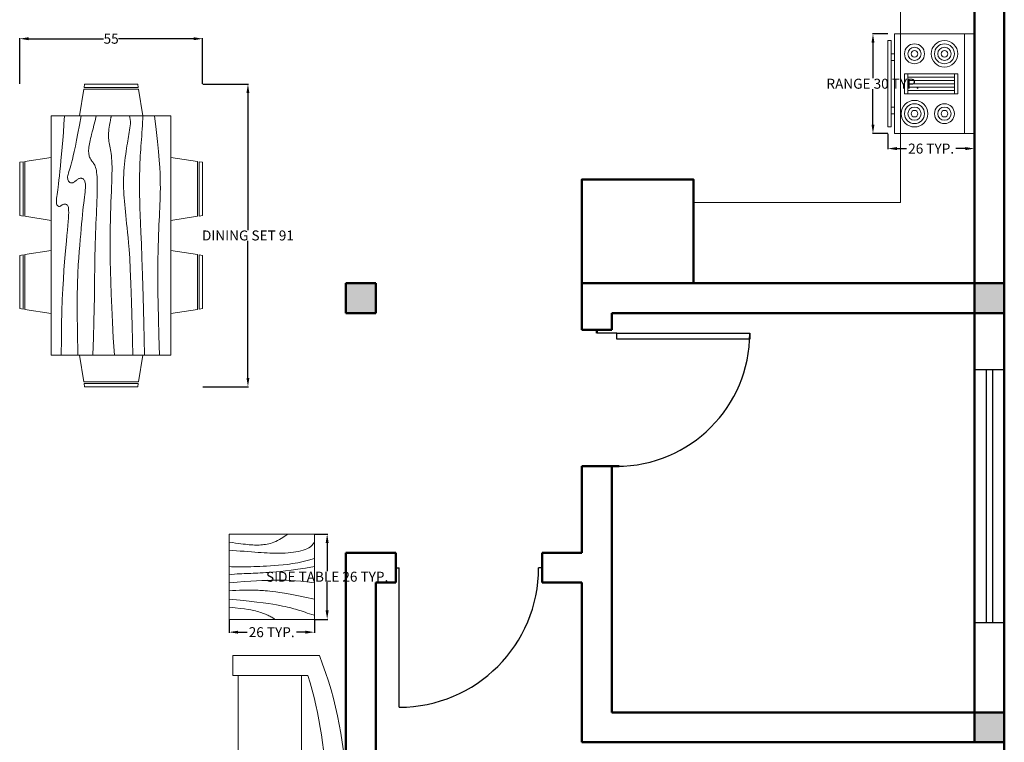
# Model space of a CAD drawing. Units: inches. Extents: x 13 to 1693, y -7 to 1519.
# Tile 3 of 10: x 387 to 683, y 360 to 577. Entities that reach past the tile are written whole.
import ezdxf

# ---------------------------------------------------------------- set-up
doc = ezdxf.new("R2010")
doc.units = ezdxf.units.IN
doc.header["$MEASUREMENT"] = 0
for name, color, linetype, lineweight in [('A-ANNO-DIMS', 2, 'Continuous', 18), ('A-DOOR', 4, 'Continuous', 25), ('A-FLOR-CASE', 5, 'Continuous', 18), ('A-FLOR-FIXT', 9, 'Continuous', 18), ('A-FURN', 8, 'Continuous', 18), ('A-GLAZ', 4, 'Continuous', 25), ('A-WALL', 7, 'Continuous', 50), ('A-WALL-PATT', 8, 'Continuous', 13)]:
    doc.layers.add(name, color=color, linetype=linetype, lineweight=lineweight)
doc.styles.get("Standard").update_dxf_attribs({"font": 'arial.ttf'})
doc.dimstyles.get("Standard").update_dxf_attribs({"dimtxt": 3, "dimasz": 2.68, "dimexe": 0.18, "dimexo": 0.0625, "dimgap": 0.09, "dimtad": 0, "dimtih": 1, "dimtoh": 1, "dimdec": 0, "dimzin": 0, "dimdsep": 46, "dimlunit": 3, "dimtxsty": 'Standard', "dimcen": 0.09, "dimadec": 0, "dimazin": 0, "dimtfac": 1, "dimtdec": 0, "dimtofl": 0, "dimtmove": 0, "dimatfit": 3, "dimfxl": 1, "dimtolj": 1, "dimtzin": 0, "dimarcsym": 0})

# ---------------------------------------------------------------- blocks, each defined once
blk = doc.blocks.new('*U6')
for p, q in [((0, 0), (0, -6)), ((40, 0), (40, -6))]:
    blk.add_line(p, q)
blk.add_lwpolyline([(0, 0), (0, 40), (1.75, 40), (1.75, 0)], close=True)
blk.add_arc((0, 0), 40, 0, 90)
blk = doc.blocks.new('Table - Square Woodgrain 42 x 42 in.')
blk.add_line((0, -42), (42, -42))
for points in [[(0, -4), (1.704, -4.2172), (3.2358, -4.4188), (4.615, -4.604), (5.8615, -4.7721), (6.9951, -4.9224), (8.0357, -5.0541), (9.0031, -5.1667), (9.9171, -5.2594), (10.7951, -5.3316), (11.6445, -5.3836), (12.4702, -5.4157), (13.277, -5.4283), (14.0698, -5.4217), (14.8535, -5.3964), (15.6331, -5.3526), (16.4133, -5.2908), (17.1986, -5.2103), (17.9913, -5.1062), (18.793, -4.9727), (19.6056, -4.8038), (20.4307, -4.5937), (21.2701, -4.3365), (22.1256, -4.0262), (22.9989, -3.6571), (23.888, -3.2272), (24.7756, -2.7516), (25.6408, -2.2491), (26.4624, -1.7387), (27.2195, -1.2395), (27.891, -0.7703), (28.456, -0.3501), (28.8934, 0.002)], [(0, -42), (0, 0), (42, 0), (42, -42)], [(0, -8), (1.8203, -8.1001), (3.6741, -8.2149), (5.5411, -8.3408), (7.4011, -8.4741), (9.2339, -8.6112), (11.0193, -8.7484), (12.7371, -8.8821), (14.3671, -9.0086), (15.8954, -9.1246), (17.3337, -9.2278), (18.6997, -9.3159), (20.0116, -9.387), (21.2871, -9.4389), (22.5442, -9.4696), (23.8008, -9.477), (25.0749, -9.459), (26.3791, -9.4137), (27.7049, -9.3403), (29.0383, -9.2382), (30.3655, -9.1068), (31.6728, -8.9455), (32.9461, -8.7535), (34.1717, -8.5304), (35.3358, -8.2756), (36.4268, -7.9863), (37.443, -7.6521), (38.3849, -7.2603), (39.253, -6.7986), (40.048, -6.2542), (40.7705, -5.6147), (41.421, -4.8674), (42, -4)], [(42, -12), (39.1784, -12.8621), (36.4519, -13.5654), (33.8246, -14.1294), (31.3004, -14.5731), (28.8832, -14.9161), (26.577, -15.1775), (24.3858, -15.3768), (22.3136, -15.5332), (20.3622, -15.6632), (18.5254, -15.7718), (16.7947, -15.8612), (15.1618, -15.9338), (13.6183, -15.9916), (12.1558, -16.0369), (10.7659, -16.0718), (9.4403, -16.0987), (8.1703, -16.1191), (6.9461, -16.1325), (5.7577, -16.1377), (4.595, -16.1335), (3.4479, -16.1188), (2.3064, -16.0924), (1.1604, -16.0532), (0, -16)], [(42, -16), (37.6529, -16.7365), (33.8802, -17.329), (30.6179, -17.7961), (27.8015, -18.1561), (25.3668, -18.4275), (23.2497, -18.6288), (21.3859, -18.7785), (19.7111, -18.8949), (18.1693, -18.9939), (16.7375, -19.0795), (15.401, -19.1534), (14.1449, -19.217), (12.9544, -19.2717), (11.8148, -19.3191), (10.7113, -19.3606), (9.6291, -19.3976), (8.5534, -19.4323), (7.47, -19.4689), (6.3643, -19.5122), (5.222, -19.5672), (4.0288, -19.6386), (2.7703, -19.7313), (1.4321, -19.8501), (0, -20)], [(0, -24), (3.9243, -23.6805), (7.4766, -23.4138), (10.6891, -23.1954), (13.5943, -23.0205), (16.2247, -22.8847), (18.6125, -22.7832), (20.7903, -22.7116), (22.7903, -22.6651), (24.6563, -22.642), (26.4764, -22.6507), (28.35, -22.7024), (30.3766, -22.8084), (32.6555, -22.98), (35.2861, -23.2283), (38.3678, -23.5645), (42, -24)], [(42, -32), (37.392, -31.017), (33.4585, -30.2231), (30.1291, -29.5949), (27.3334, -29.109), (25.0009, -28.742), (23.0612, -28.4707), (21.4439, -28.2716), (20.0786, -28.1215), (18.8998, -28.0002), (17.8609, -27.9014), (16.9206, -27.8219), (16.0371, -27.7588), (15.1691, -27.709), (14.2748, -27.6693), (13.3128, -27.6368), (12.2415, -27.6083), (11.0295, -27.5824), (9.6867, -27.5643), (8.233, -27.5608), (6.6884, -27.5787), (5.0728, -27.6248), (3.4062, -27.7058), (1.7086, -27.8286), (0, -28)], [(0, -32), (5.4026, -32.5358), (9.9494, -33.019), (13.7424, -33.4553), (16.8834, -33.8505), (19.4743, -34.2106), (21.6171, -34.5413), (23.4136, -34.8486), (24.9657, -35.1382), (26.3614, -35.4156), (27.6332, -35.6841), (28.7995, -35.9467), (29.8788, -36.2064), (30.8897, -36.4661), (31.8507, -36.7288), (32.7802, -36.9973), (33.6968, -37.2747), (34.6175, -37.5635), (35.5531, -37.8651), (36.5128, -38.1805), (37.506, -38.5108), (38.5421, -38.8568), (39.6302, -39.2197), (40.7797, -39.6004), (42, -40)], [(0, -36), (3.0098, -36.2857), (5.5354, -36.5643), (7.6368, -36.8359), (9.374, -37.1009), (10.807, -37.3597), (11.9957, -37.6126), (13.0002, -37.8599), (13.8804, -38.102), (14.6874, -38.3393), (15.4365, -38.5729), (16.1338, -38.8041), (16.7858, -39.0341), (17.3987, -39.264), (17.9787, -39.4952), (18.5322, -39.7288), (19.0655, -39.9662), (19.5832, -40.2081), (20.0842, -40.4544), (20.5657, -40.7046), (21.0249, -40.9581), (21.459, -41.2144), (21.8653, -41.4731), (22.2409, -41.7335), (22.5831, -41.9951)]]:
    blk.add_lwpolyline(points)
blk = doc.blocks.new('Sofa - Roundback 7 ft.')
for p, q in [((-12.00002, -32.4421), (-12.00003, -6.5971)), ((11.99997, -32.4421), (11.99998, -6.5971)), ((-36.000027, -34), (-36.000027, -11.4696)), ((35.99998, -34), (35.99998, -11.4696)), ((-35.999844, -13.3819), (35.9998, -13.3819)), ((-36.000027, -32.4421), (35.99998, -32.4421))]:
    blk.add_line(p, q)
for points in [[(-36.000027, -34), (-42.000027, -34), (-42.000027, -8)], [(41.99998, -8), (41.99998, -34), (35.99998, -34)]]:
    blk.add_lwpolyline(points)
for centre, radius, start, end in [((0, -114.25), 114.25, 68.43141, 111.5686), ((-0.00001, -127.1968), 121.1968, 72.72033, 107.2797)]:
    blk.add_arc(centre, radius, start, end)
blk = doc.blocks.new('Dining Set - 36 x 72 in.')
for p, q in [((-22, 27.5), (-22.1562, 26.50042)), ((-22, 27.5), (-6, 27.5)), ((-5.8437, 26.49966), (-6, 27.5)), ((6, 27.5), (5.8438, 26.50042)), ((6, 27.5), (22, 27.5)), ((22.1563, 26.49966), (22, 27.5)), ((-22.2343, 26.00059), (-23.4847, 17.99762)), ((-22.2304, 26), (-5.7608, 26)), ((-5.8416, 26.5), (-22.1534, 26.5)), ((-4.5152, 17.99762), (-5.7655, 25.99926)), ((5.7657, 26.00059), (4.5153, 17.99762)), ((5.7696, 26), (22.2392, 26)), ((22.1584, 26.5), (5.8466, 26.5)), ((23.4848, 17.99762), (22.2345, 25.99926)), ((36, 18), (-36, 18)), ((-36, 18), (-36, -18)), ((36, -18), (36, 18)), ((-44.0006, 8.23428), (-35.9976, 9.48474)), ((44.0006, 8.23428), (35.9976, 9.48474)), ((-45.5, 8), (-44.5004, 8.15617)), ((-45.5, 8), (-45.5, -8)), ((-44.5, -8.15843), (-44.5, 8.15338)), ((-44, 8.23041), (-44, -8.23915)), ((44, 8.23041), (44, -8.23915)), ((44.5, -8.15843), (44.5, 8.15338)), ((45.5, 8), (44.5005, 8.15617)), ((45.5, 8), (45.5, -8)), ((-44.4997, -8.15631), (-45.5, -8)), ((-35.9976, -9.48476), (-43.9993, -8.2345)), ((35.9976, -9.48476), (43.9993, -8.2345)), ((44.4997, -8.15631), (45.5, -8)), ((-36, -18), (36, -18)), ((-22.2343, -26.0006), (-23.4847, -17.99762)), ((-4.5152, -17.99762), (-5.7655, -25.99928)), ((5.7657, -26.0006), (4.5153, -17.99762)), ((23.4848, -17.99762), (22.2345, -25.99928)), ((-22.2304, -26), (-5.7608, -26)), ((-22, -27.5), (-22.1562, -26.50044)), ((-5.8416, -26.5), (-22.1534, -26.5)), ((-5.8437, -26.49967), (-6, -27.5)), ((5.7696, -26), (22.2392, -26)), ((6, -27.5), (5.8438, -26.50044)), ((22.1584, -26.5), (5.8466, -26.5)), ((22.1563, -26.49967), (22, -27.5)), ((-22, -27.5), (-6, -27.5)), ((6, -27.5), (22, -27.5))]:
    blk.add_line(p, q)
for points in [[(-36, 15), (-31.1772, 14.97754), (-26.8079, 14.91406), (-22.8538, 14.81543), (-19.276, 14.6875), (-16.0362, 14.53613), (-13.0957, 14.36718), (-10.4159, 14.18652), (-7.9583, 14), (-5.6904, 13.81315), (-3.6035, 13.63021), (-1.6954, 13.45508), (0.0365, 13.29166), (1.5945, 13.14388), (2.9811, 13.01562), (4.1988, 12.9108), (5.25, 12.83333), (6.1393, 12.78613), (6.8802, 12.76823), (7.4883, 12.77767), (7.9792, 12.8125), (8.3685, 12.87077), (8.6719, 12.95052), (8.9049, 13.0498), (9.0833, 13.16666), (9.2205, 13.29899), (9.3216, 13.44401), (9.3895, 13.59879), (9.4271, 13.76041), (9.4373, 13.92594), (9.4232, 14.09245), (9.3875, 14.257), (9.3333, 14.41666), (9.2638, 14.56917), (9.1836, 14.71484), (9.0975, 14.85465), (9.0104, 14.98958), (8.9272, 15.1206), (8.8529, 15.2487), (8.7922, 15.37483), (8.75, 15.5), (8.7305, 15.62467), (8.7344, 15.74739), (8.7617, 15.86621), (8.8125, 15.97916), (8.8867, 16.08431), (8.9844, 16.17968), (9.1055, 16.26334), (9.25, 16.33333), (9.4189, 16.38802), (9.6172, 16.42708), (9.8506, 16.45052), (10.125, 16.45833), (10.4463, 16.45052), (10.8203, 16.42708), (11.2529, 16.38802), (11.75, 16.33333), (12.3184, 16.26318), (12.9694, 16.17838), (13.7151, 16.07991), (14.5677, 15.96875), (15.5395, 15.84586), (16.6426, 15.71224), (17.8893, 15.56884), (19.2917, 15.41666), (20.859, 15.25667), (22.5879, 15.08984), (24.4721, 14.91715), (26.5052, 14.73958), (28.6809, 14.5581), (30.9929, 14.3737), (33.4347, 14.18733), (36, 14)], [(-36, 10), (-28.9766, 10.14274), (-23.1725, 10.20442), (-18.4241, 10.19775), (-14.5677, 10.13541), (-11.4399, 10.03011), (-8.877, 9.89453), (-6.7154, 9.74137), (-4.7917, 9.58333), (-2.9698, 9.43082), (-1.2246, 9.28515), (0.4415, 9.14534), (2.026, 9.01041), (3.5266, 8.87939), (4.9408, 8.7513), (6.266, 8.62516), (7.5, 8.5), (8.6411, 8.37549), (9.6914, 8.2539), (10.6538, 8.13818), (11.5312, 8.03125), (12.3267, 7.93603), (13.043, 7.85547), (13.6831, 7.79248), (14.25, 7.75), (14.7471, 7.7303), (15.1797, 7.73307), (15.5537, 7.75732), (15.875, 7.80208), (16.1494, 7.86637), (16.3828, 7.94922), (16.5811, 8.04964), (16.75, 8.16666), (16.8944, 8.29915), (17.0143, 8.44531), (17.1089, 8.60319), (17.1771, 8.77083), (17.218, 8.94629), (17.2305, 9.1276), (17.2137, 9.31282), (17.1667, 9.5), (17.0895, 9.6875), (16.987, 9.875), (16.8649, 10.0625), (16.7292, 10.25), (16.5856, 10.4375), (16.4401, 10.625), (16.2985, 10.8125), (16.1667, 11), (16.05, 11.18733), (15.9518, 11.3737), (15.8752, 11.5581), (15.8229, 11.73958), (15.798, 11.91715), (15.8034, 12.08984), (15.842, 12.25667), (15.9167, 12.41666), (16.0295, 12.56836), (16.1784, 12.70833), (16.3605, 12.83268), (16.5729, 12.9375), (16.8127, 13.01888), (17.0768, 13.07291), (17.3625, 13.0957), (17.6667, 13.08333), (17.9894, 13.03312), (18.3418, 12.94726), (18.7382, 12.82918), (19.1927, 12.68229), (19.7195, 12.51001), (20.3327, 12.31575), (21.0465, 12.10294), (21.875, 11.875), (22.8357, 11.63354), (23.959, 11.37304), (25.2786, 11.08618), (26.8282, 10.76562), (28.6414, 10.40405), (30.752, 9.99414), (33.1936, 9.52856), (36, 9)], [(-36, 5.5), (-30.7157, 5.3348), (-26.069, 5.20963), (-21.9946, 5.11767), (-18.4271, 5.05208), (-15.3009, 5.00602), (-12.5508, 4.97265), (-10.1112, 4.94515), (-7.9167, 4.91666), (-5.909, 4.88167), (-4.0586, 4.83984), (-2.3429, 4.79215), (-0.7396, 4.73958), (0.7739, 4.6831), (2.22, 4.6237), (3.6213, 4.56233), (5, 4.5), (6.373, 4.43782), (7.7344, 4.3776), (9.0723, 4.32129), (10.375, 4.27083), (11.6309, 4.22819), (12.8281, 4.19531), (13.9551, 4.17415), (15, 4.16666), (15.954, 4.17448), (16.819, 4.19791), (17.6001, 4.23698), (18.3021, 4.29166), (18.9299, 4.36198), (19.4883, 4.44791), (19.9823, 4.54948), (20.4167, 4.66666), (20.7969, 4.79899), (21.1302, 4.94401), (21.4245, 5.09879), (21.6875, 5.26041), (21.9271, 5.42594), (22.1511, 5.59245), (22.3672, 5.757), (22.5834, 5.91666), (22.8065, 6.06868), (23.0404, 6.21093), (23.2879, 6.34147), (23.5521, 6.45833), (23.8358, 6.55957), (24.142, 6.64323), (24.4735, 6.70735), (24.8334, 6.75), (25.2235, 6.76969), (25.642, 6.76692), (26.0858, 6.74267), (26.5521, 6.69791), (27.0379, 6.63362), (27.5404, 6.55078), (28.0565, 6.45036), (28.5834, 6.33333), (29.1242, 6.19987), (29.7071, 6.04687), (30.3661, 5.87044), (31.1354, 5.66666), (32.0493, 5.43164), (33.142, 5.16146), (34.4475, 4.85221), (36, 4.5)], [(-36, -1), (-30.7915, -0.6591), (-26.0195, -0.38216), (-21.6519, -0.16284), (-17.6563, 0.00521), (-14.0005, 0.12833), (-10.6523, 0.21289), (-7.5796, 0.26522), (-4.75, 0.29166), (-2.134, 0.29793), (0.2878, 0.28711), (2.5317, 0.26163), (4.6146, 0.22396), (6.5529, 0.17651), (8.3633, 0.12174), (10.0623, 0.06209), (11.6667, 0), (13.1899, -0.06201), (14.6341, -0.1211), (15.9982, -0.17432), (17.2813, -0.21875), (18.4823, -0.25147), (19.6003, -0.26953), (20.6343, -0.27002), (21.5834, -0.25), (22.4481, -0.20768), (23.2357, -0.14584), (23.9549, -0.06836), (24.6146, 0.02083), (25.2235, 0.11784), (25.7904, 0.21875), (26.3241, 0.31966), (26.8334, 0.41666), (27.3265, 0.50618), (27.8099, 0.58593), (28.2894, 0.65397), (28.7709, 0.70833), (29.2601, 0.74707), (29.763, 0.76823), (30.2855, 0.76985), (30.8334, 0.75), (31.4088, 0.70784), (31.9994, 0.64713), (32.589, 0.57275), (33.1615, 0.48958), (33.7008, 0.4025), (34.1908, 0.3164), (34.6153, 0.23616), (34.9584, 0.16666), (35.2099, 0.11165), (35.3848, 0.07031), (35.504, 0.04069), (35.5886, 0.02083), (35.6594, 0.00879), (35.7377, 0.0026), (35.8442, 0.00032), (36, 0)], [(-36, -6.5), (-27.1843, -6.31267), (-20.084, -6.1263), (-14.469, -5.9419), (-10.1094, -5.76042), (-6.7752, -5.58285), (-4.2363, -5.41016), (-2.2629, -5.24333), (-0.625, -5.08334), (0.8708, -4.93099), (2.2715, -4.78646), (3.5872, -4.64974), (4.8281, -4.52084), (6.0046, -4.39974), (7.127, -4.28646), (8.2053, -4.18099), (9.25, -4.08334), (10.2705, -3.99382), (11.2734, -3.91407), (12.2647, -3.84603), (13.25, -3.79167), (14.2354, -3.75293), (15.2266, -3.73177), (16.2295, -3.73015), (17.25, -3.75), (18.2912, -3.79248), (19.3451, -3.85547), (20.4009, -3.93604), (21.4479, -4.03125), (22.4754, -4.13819), (23.4727, -4.25391), (24.4289, -4.37549), (25.3334, -4.5), (26.1785, -4.62492), (26.9694, -4.74935), (27.7145, -4.87281), (28.4219, -4.99479), (29.1, -5.11483), (29.7572, -5.23242), (30.4016, -5.34709), (31.0417, -5.45834), (31.6837, -5.56437), (32.3262, -5.65821), (32.9658, -5.73153), (33.599, -5.77604), (34.2224, -5.78345), (34.8327, -5.74545), (35.4264, -5.65373), (36, -5.5)], [(-36, -10), (-26.4022, -9.81299), (-18.4675, -9.62891), (-11.9839, -9.45069), (-6.7396, -9.28125), (-2.5226, -9.12354), (0.8789, -8.98047), (3.6769, -8.85498), (6.0833, -8.75), (8.2767, -8.66765), (10.3021, -8.60677), (12.1712, -8.56543), (13.8958, -8.54167), (15.4876, -8.53353), (16.9583, -8.53907), (18.3197, -8.55632), (19.5834, -8.58334), (20.7616, -8.61841), (21.8685, -8.66081), (22.9188, -8.71004), (23.9271, -8.76563), (24.9081, -8.82707), (25.8763, -8.89388), (26.8465, -8.96558), (27.8334, -9.04167), (28.8474, -9.12118), (29.8828, -9.20117), (30.93, -9.27824), (31.9792, -9.34896), (33.0205, -9.40991), (34.0443, -9.45768), (35.0407, -9.48885), (36, -9.5)], [(-36, -14.5), (-30.0881, -14.33513), (-25.0332, -14.21224), (-20.7312, -14.12647), (-17.0781, -14.07292), (-13.97, -14.04671), (-11.3027, -14.04297), (-8.9724, -14.05681), (-6.875, -14.08334), (-4.9224, -14.11833), (-3.0905, -14.16016), (-1.3709, -14.20785), (0.2448, -14.26042), (1.7647, -14.3169), (3.1973, -14.3763), (4.5507, -14.43767), (5.8333, -14.5), (7.0554, -14.5621), (8.235, -14.62175), (9.3922, -14.67652), (10.5469, -14.72396), (11.7192, -14.76164), (12.929, -14.78711), (14.1965, -14.79794), (15.5417, -14.79167), (16.9933, -14.76424), (18.6152, -14.70508), (20.4804, -14.60197), (22.6615, -14.44271), (25.2312, -14.21509), (28.2624, -13.9069), (31.8277, -13.50594), (36, -13)]]:
    blk.add_lwpolyline(points)
blk = doc.blocks.new('Range-Oven - 30 in top')
for p, q in [((0, -3), (30, -3)), ((12, -6), (18, -6)), ((13, -20), (13, -6)), ((14, -6), (14, -20)), ((15, -20), (15, -6)), ((16, -6), (16, -20)), ((17, -20), (17, -6)), ((18, -20), (12, -20)), ((6, -24), (6, -25)), ((8, -25), (8, -24)), ((22, -25), (22, -24)), ((24, -24), (24, -25))]:
    blk.add_line(p, q)
for points in [[(0, -24), (0, 0), (30, 0), (30, -24)], [(12, -21), (12, -5), (18, -5), (18, -21)], [(2, -26), (2, -25), (28, -25), (28, -26)]]:
    blk.add_lwpolyline(points, close=True)
for centre, radius in [((6, -9), 4), ((6, -9), 3), ((6, -9), 2), ((6, -9), 1), ((24, -9), 3), ((24, -9), 2), ((24, -9), 1), ((24, -18), 4), ((6, -18), 3), ((6, -18), 2), ((6, -18), 1), ((24, -18), 3), ((24, -18), 2), ((24, -18), 1)]:
    blk.add_circle(centre, radius)
blk = doc.blocks.new('WIN-76')
for p, q in [((0, 9), (0, 0)), ((76.02, 9), (76.02, 0)), ((0, 5.5), (76.02, 5.5)), ((0, 3.5), (76.02, 3.5))]:
    blk.add_line(p, q)
blk = doc.blocks.new('DOOR-42')
for p, q in [((0, 41.95), (1, 41.95)), ((1, 0), (1, 41.95)), ((43.95, 41.95), (42.95, 41.95))]:
    blk.add_line(p, q)
blk.add_arc((1, 41.95), 41.95, 270, 0)
blk = doc.blocks.new('*D54')
at = {"layer": 'A-ANNO-DIMS', "color": 0, "lineweight": -2, "transparency": 16777216}
for p, q in [((476, 422.76), (479.97, 422.76)), ((479.79, 420.08), (479.79, 411.58)), ((479.79, 399.79), (479.79, 408.29)), ((476, 397.11), (479.97, 397.11))]:
    blk.add_line(p, q, dxfattribs=at)
at = {"layer": 'A-ANNO-DIMS', "color": 0, "transparency": 16777216}
for points in [[(479.34, 420.08), (480.24, 420.08), (479.79, 422.76)], [(479.34, 399.79), (480.24, 399.79), (479.79, 397.11)]]:
    blk.add_solid(points, dxfattribs=at)
at = {"layer": 'Defpoints', "color": 0, "transparency": 16777216}
for p in [(475.94, 422.76), (479.79, 422.76), (475.94, 397.11)]:
    blk.add_point(p, dxfattribs=at)
at = {"layer": 'A-ANNO-DIMS', "color": 0, "transparency": 16777216, "insert": (479.79, 409.93), "char_height": 3, "attachment_point": 5}
blk.add_mtext('\\A1;SIDE TABLE 26 TYP.', dxfattribs=at)
blk = doc.blocks.new('*D55')
at = {"layer": 'A-ANNO-DIMS', "color": 0, "lineweight": -2, "transparency": 16777216}
for p, q in [((450.28, 397.04), (450.28, 393.08)), ((475.94, 397.04), (475.94, 393.08)), ((452.96, 393.26), (455.69, 393.26)), ((473.26, 393.26), (470.53, 393.26))]:
    blk.add_line(p, q, dxfattribs=at)
at = {"layer": 'A-ANNO-DIMS', "color": 0, "transparency": 16777216}
for points in [[(452.96, 393.7), (452.96, 392.81), (450.28, 393.26)], [(473.26, 393.7), (473.26, 392.81), (475.94, 393.26)]]:
    blk.add_solid(points, dxfattribs=at)
at = {"layer": 'Defpoints', "color": 0, "transparency": 16777216}
for p in [(450.28, 397.11), (475.94, 397.11), (475.94, 393.26)]:
    blk.add_point(p, dxfattribs=at)
at = {"layer": 'A-ANNO-DIMS', "color": 0, "transparency": 16777216, "insert": (463.11, 393.26), "char_height": 3, "attachment_point": 5}
blk.add_mtext('\\A1;26 TYP.', dxfattribs=at)
blk = doc.blocks.new('*D62')
at = {"layer": 'A-ANNO-DIMS', "color": 0, "lineweight": -2, "transparency": 16777216}
for p, q in [((648.39, 573.15), (643.77, 573.15)), ((643.95, 570.47), (643.95, 559.79)), ((643.95, 545.83), (643.95, 556.51)), ((648.39, 543.15), (643.77, 543.15))]:
    blk.add_line(p, q, dxfattribs=at)
at = {"layer": 'A-ANNO-DIMS', "color": 0, "transparency": 16777216}
for points in [[(643.51, 570.47), (644.4, 570.47), (643.95, 573.15)], [(643.51, 545.83), (644.4, 545.83), (643.95, 543.15)]]:
    blk.add_solid(points, dxfattribs=at)
at = {"layer": 'Defpoints', "color": 0, "transparency": 16777216}
for p in [(648.45, 573.15), (643.95, 543.15), (648.45, 543.15)]:
    blk.add_point(p, dxfattribs=at)
at = {"layer": 'A-ANNO-DIMS', "color": 0, "transparency": 16777216, "insert": (643.95, 558.15), "char_height": 3, "attachment_point": 5}
blk.add_mtext('\\A1;RANGE 30 TYP.', dxfattribs=at)
blk = doc.blocks.new('*D63')
at = {"layer": 'A-ANNO-DIMS', "color": 0, "lineweight": -2, "transparency": 16777216}
for p, q in [((648.45, 543.09), (648.45, 538.47)), ((674.45, 543.09), (674.45, 538.47)), ((651.13, 538.65), (654.04, 538.65)), ((671.77, 538.65), (668.87, 538.65))]:
    blk.add_line(p, q, dxfattribs=at)
at = {"layer": 'A-ANNO-DIMS', "color": 0, "transparency": 16777216}
for points in [[(651.13, 539.1), (651.13, 538.2), (648.45, 538.65)], [(671.77, 539.1), (671.77, 538.2), (674.45, 538.65)]]:
    blk.add_solid(points, dxfattribs=at)
at = {"layer": 'Defpoints', "color": 0, "transparency": 16777216}
for p in [(648.45, 543.15), (674.45, 543.15), (674.45, 538.65)]:
    blk.add_point(p, dxfattribs=at)
at = {"layer": 'A-ANNO-DIMS', "color": 0, "transparency": 16777216, "insert": (661.45, 538.65), "char_height": 3, "attachment_point": 5}
blk.add_mtext('\\A1;26 TYP.', dxfattribs=at)
blk = doc.blocks.new('*D74')
at = {"layer": 'A-ANNO-DIMS', "color": 0, "lineweight": -2, "transparency": 16777216}
for p, q in [((442.38, 558.03), (456.15, 558.03)), ((455.97, 555.35), (455.97, 514.17)), ((455.97, 469.71), (455.97, 510.89)), ((442.38, 467.03), (456.15, 467.03))]:
    blk.add_line(p, q, dxfattribs=at)
at = {"layer": 'A-ANNO-DIMS', "color": 0, "transparency": 16777216}
for points in [[(455.52, 555.35), (456.41, 555.35), (455.97, 558.03)], [(455.52, 469.71), (456.41, 469.71), (455.97, 467.03)]]:
    blk.add_solid(points, dxfattribs=at)
at = {"layer": 'Defpoints', "color": 0, "transparency": 16777216}
for p in [(442.32, 558.03), (455.97, 558.03), (442.32, 467.03)]:
    blk.add_point(p, dxfattribs=at)
at = {"layer": 'A-ANNO-DIMS', "color": 0, "transparency": 16777216, "insert": (455.97, 512.53), "char_height": 3, "attachment_point": 5}
blk.add_mtext('\\A1;DINING SET 91', dxfattribs=at)
blk = doc.blocks.new('*D75')
at = {"layer": 'A-ANNO-DIMS', "color": 0, "lineweight": -2, "transparency": 16777216}
for p, q in [((387.32, 558.1), (387.32, 571.86)), ((390, 571.68), (412.57, 571.68)), ((439.64, 571.68), (417.07, 571.68)), ((442.32, 558.1), (442.32, 571.86))]:
    blk.add_line(p, q, dxfattribs=at)
at = {"layer": 'A-ANNO-DIMS', "color": 0, "transparency": 16777216}
for points in [[(390, 572.13), (390, 571.24), (387.32, 571.68)], [(439.64, 572.13), (439.64, 571.24), (442.32, 571.68)]]:
    blk.add_solid(points, dxfattribs=at)
at = {"layer": 'Defpoints', "color": 0, "transparency": 16777216}
for p in [(387.32, 571.68), (387.32, 558.03), (442.32, 558.03)]:
    blk.add_point(p, dxfattribs=at)
at = {"layer": 'A-ANNO-DIMS', "color": 0, "transparency": 16777216, "insert": (414.82, 571.68), "char_height": 3, "attachment_point": 5}
blk.add_mtext('\\A1;55', dxfattribs=at)

msp = doc.modelspace()

# ---------------------------------------------------------------- hatches: boundary and pattern name
at = {"layer": 'A-WALL-PATT'}
h = msp.add_hatch(color=256, dxfattribs=at)
h.dxf.hatch_style = 1
h.paths.add_polyline_path([(683.45, 735.15), (674.45, 735.15), (674.45, 726.15), (683.45, 726.15)])
h.paths.add_polyline_path([(683.45, 657.15), (674.45, 657.15), (674.45, 648.15), (683.45, 648.15)])
h.paths.add_polyline_path([(494.45, 498.15), (485.45, 498.15), (485.45, 489.15), (494.45, 489.15)])
h.paths.add_polyline_path([(683.45, 498.15), (674.45, 498.15), (674.45, 489.15), (683.45, 489.15)])
h.paths.add_polyline_path([(494.45, 222.15), (485.45, 222.15), (485.45, 213.15), (494.45, 213.15)])
h.paths.add_polyline_path([(683.45, 369.15), (674.45, 369.15), (674.45, 360.15), (683.45, 360.15)])

# ---------------------------------------------------------------- linework, layer by layer
at = {"layer": 'A-FLOR-CASE'}
for p, q in [((652.22, 620.17), (652.22, 522.4)), ((652.22, 522.4), (589.95, 522.4))]:
    msp.add_line(p, q, dxfattribs=at)
at = {"layer": 'A-WALL'}
for p, q in [((683.45, 147.15), (683.45, 735.15)), ((674.45, 498.15), (674.45, 648.15)), ((485.45, 489.15), (485.45, 498.15)), ((494.45, 498.15), (485.45, 498.15)), ((494.45, 489.15), (494.45, 498.15)), ((674.45, 498.15), (556.41, 498.15)), ((556.41, 498.15), (556.41, 484.15)), ((674.45, 489.15), (674.45, 498.15)), ((683.45, 498.15), (674.45, 498.15)), ((683.45, 489.15), (683.45, 498.15)), ((494.45, 489.15), (485.45, 489.15)), ((674.45, 489.15), (565.41, 489.15)), ((565.41, 489.15), (565.41, 484.15)), ((674.45, 369.15), (674.45, 489.15)), ((683.45, 489.15), (674.45, 489.15)), ((556.41, 484.15), (565.41, 484.15)), ((560.91, 484.15), (560.91, 483.15)), ((556.41, 443.15), (565.41, 443.15)), ((556.41, 443.15), (556.41, 417.15)), ((567.62, 443.15), (558.62, 443.15)), ((565.41, 443.15), (565.41, 369.15)), ((500.45, 417.15), (485.45, 417.15)), ((485.45, 213.15), (485.45, 417.15)), ((500.45, 408.15), (500.45, 417.15)), ((556.41, 417.15), (544.41, 417.15)), ((544.41, 408.15), (544.41, 417.15)), ((500.45, 408.15), (494.45, 408.15)), ((494.45, 213.15), (494.45, 408.15)), ((556.41, 408.15), (544.41, 408.15)), ((556.41, 408.15), (556.41, 360.15)), ((674.45, 369.15), (565.41, 369.15)), ((674.45, 360.15), (556.41, 360.15))]:
    msp.add_line(p, q, dxfattribs=at)
for points in [[(556.41, 498.15), (589.95, 498.15), (589.95, 529.39), (556.41, 529.39)], [(674.45, 369.15), (683.45, 369.15), (683.45, 360.15), (674.45, 360.15)]]:
    msp.add_lwpolyline(points, close=True, dxfattribs=at)

# ---------------------------------------------------------------- block references
at = {"layer": 'A-DOOR', "rotation": 270}
msp.add_blockref('*U6', (566.91, 483.15), dxfattribs=at)
at = {"layer": 'A-DOOR'}
msp.add_blockref('DOOR-42', (500.45, 370.7), dxfattribs=at)
at = {"layer": 'A-FLOR-FIXT', "rotation": 270}
msp.add_blockref('Range-Oven - 30 in top', (674.45, 573.15), dxfattribs=at)
at = {"layer": 'A-FURN'}
for name, p, rotation in [('Dining Set - 36 x 72 in.', (414.82, 512.53), 90.00000000000003), ('Sofa - Roundback 7 ft.', (485.45, 344.21), 270)]:
    msp.add_blockref(name, p, dxfattribs=dict(at, rotation=rotation))
at = {"layer": 'A-FURN', "xscale": 0.6108650724074032, "yscale": 0.6108650724074032, "zscale": 0.6108650724074032}
msp.add_blockref('Table - Square Woodgrain 42 x 42 in.', (450.28, 422.76), dxfattribs=at)
at = {"layer": 'A-GLAZ', "rotation": 270}
msp.add_blockref('WIN-76', (674.45, 472.13), dxfattribs=at)

# ---------------------------------------------------------------- dimensions: what is measured, and where the dimension line sits
at = {"layer": 'A-ANNO-DIMS'}
dim = msp.add_linear_dim(base=(387.32, 571.68), p1=(442.32, 558.03), p2=(387.32, 558.03), angle=180, dimstyle='Standard', override={"dimdec": 0, "dimlfac": 1, "dimrnd": 0, "dimzin": 0, "dimdsep": 46, "dimlunit": 2}, dxfattribs=at)
dim.commit()
dim.dimension.update_dxf_attribs({"geometry": '*D75', "text_midpoint": (414.82, 571.68)})
for base, p1, p2, angle, text, picture, middle in [((643.95, 543.15), (648.45, 573.15), (648.45, 543.15), 270, 'RANGE <> TYP.', '*D62', (643.95, 558.15)), ((455.97, 558.03), (442.32, 467.03), (442.32, 558.03), 90, 'DINING SET <>', '*D74', (455.97, 512.53)), ((479.79, 422.76), (475.94, 397.11), (475.94, 422.76), 90, 'SIDE TABLE <> TYP.', '*D54', (479.79, 409.93))]:
    dim = msp.add_linear_dim(base=base, p1=p1, p2=p2, angle=angle, text=text, dimstyle='Standard', override={"dimdec": 0, "dimlfac": 1, "dimrnd": 0, "dimzin": 0, "dimdsep": 46, "dimlunit": 2}, dxfattribs=at)
    dim.commit()
    dim.dimension.update_dxf_attribs({"geometry": picture, "text_midpoint": middle})
for base, p1, p2, picture, middle in [((674.45, 538.65), (648.45, 543.15), (674.45, 543.15), '*D63', (661.45, 538.65)), ((475.94, 393.26), (450.28, 397.11), (475.94, 397.11), '*D55', (463.11, 393.26))]:
    dim = msp.add_linear_dim(base=base, p1=p1, p2=p2, text='<> TYP.', dimstyle='Standard', override={"dimdec": 0, "dimlfac": 1, "dimrnd": 0, "dimzin": 0, "dimdsep": 46, "dimlunit": 2}, dxfattribs=at)
    dim.commit()
    dim.dimension.update_dxf_attribs({"geometry": picture, "text_midpoint": middle})

doc.saveas('drawing.dxf')
